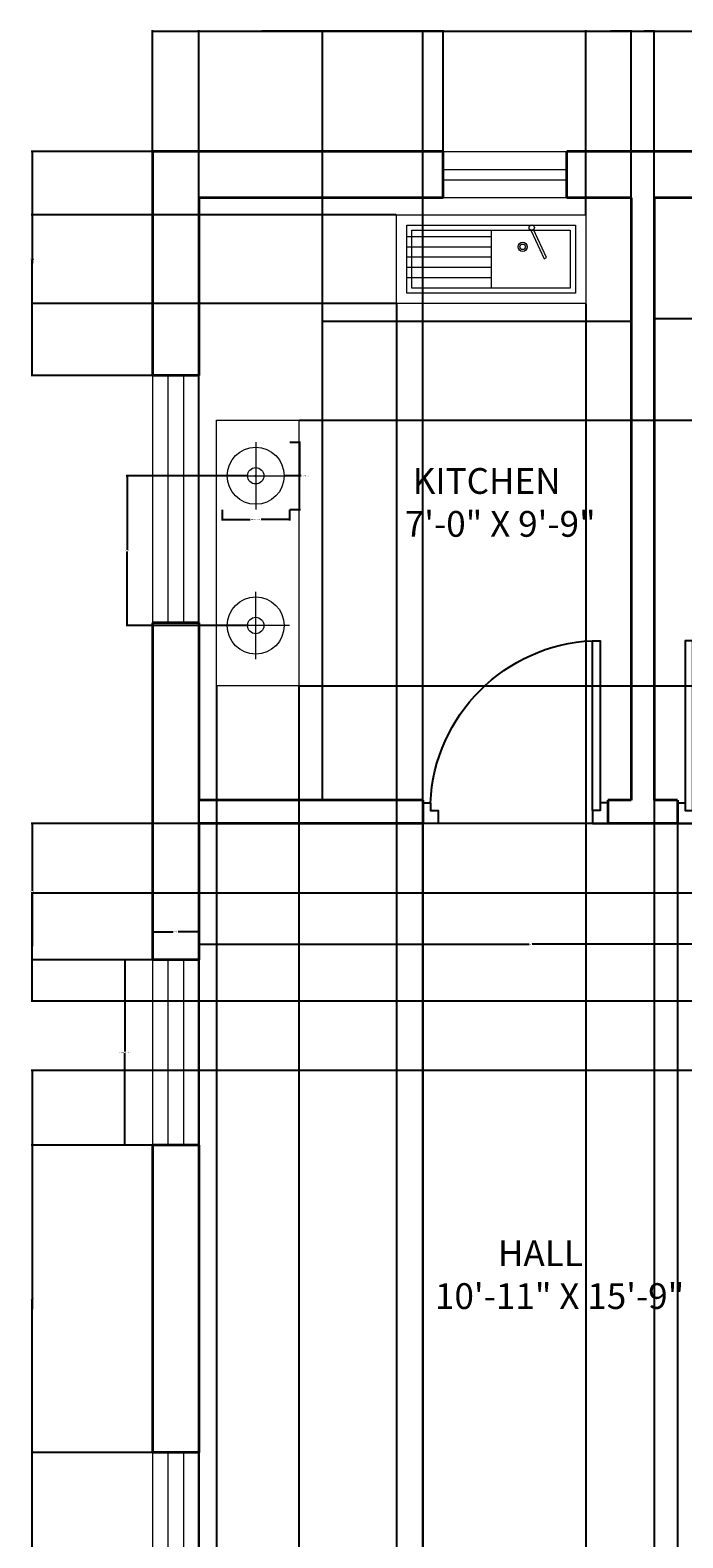
# Model space of a CAD drawing. Units: inches. Extents: x 324 to 662, y 102 to 605.
# Tile 3 of 4: x 324 to 451, y 313 to 605. Entities that reach past the tile are written whole.
import ezdxf

# ---------------------------------------------------------------- set-up
doc = ezdxf.new("R2010")
doc.units = ezdxf.units.IN
for name, color, linetype, lineweight in [('A-ANNO-DIMS', 2, 'Continuous', 18), ('A-AREA-IDEN', 7, 'Continuous', 25), ('A-EQPM', 8, 'Continuous', 18), ('A-FLOR-CASE', 8, 'Continuous', 25), ('A-FLOR-FIXT', 8, 'Continuous', 18), ('door', 82, 'Continuous', 25), ('ventilator', 20, 'Continuous', 18), ('wall', 7, 'Continuous', 35), ('window', 50, 'Continuous', 18)]:
    doc.layers.add(name, color=color, linetype=linetype, lineweight=lineweight)
doc.styles.get("Standard").update_dxf_attribs({"font": 'arial.ttf'})
doc.dimstyles.get("Standard").update_dxf_attribs({"dimtxt": 0.18, "dimasz": 0.18, "dimexe": 0.18, "dimexo": 0.0625, "dimgap": 0.09, "dimtad": 0, "dimtih": 1, "dimtoh": 1, "dimdec": 4, "dimzin": 0, "dimdsep": 46, "dimtxsty": 'Standard', "dimcen": 0.09, "dimadec": 0, "dimazin": 0, "dimtfac": 1, "dimtdec": 4, "dimtofl": 0, "dimtmove": 0, "dimatfit": 3, "dimfxl": 1, "dimtolj": 1, "dimtzin": 0, "dimarcsym": 0})

# ---------------------------------------------------------------- blocks, each defined once
blk = doc.blocks.new('w1')
at = {"layer": 'window'}
for p, q in [((719.66, 290.3), (719.66, 242.3)), ((722.66, 290.3), (722.66, 242.3))]:
    blk.add_line(p, q, dxfattribs=at)
blk.add_lwpolyline([(716.66, 242.3), (725.66, 242.3), (725.66, 290.3), (716.66, 290.3)], close=True, dxfattribs=at)
blk = doc.blocks.new('w2')
at = {"layer": 'window'}
for p, q in [((765.26, 316.2), (765.26, 280.2)), ((768.26, 316.2), (768.26, 280.2))]:
    blk.add_line(p, q, dxfattribs=at)
blk.add_lwpolyline([(762.26, 280.2), (771.26, 280.2), (771.26, 316.2), (762.26, 316.2)], close=True, dxfattribs=at)
blk = doc.blocks.new('d1')
at = {"layer": 'door'}
blk.add_line((825.6, 316.36), (861.6, 316.36), dxfattribs=at)
blk.add_lwpolyline([(827.1, 318.86), (828.6, 318.86), (828.6, 351.86), (827.1, 351.86)], close=True, dxfattribs=at)
for points in [[(828.6, 316.36), (825.6, 316.36), (825.6, 320.36), (827.1, 320.36), (827.1, 318.86), (828.6, 318.86), (828.6, 316.36)], [(858.6, 316.36), (861.6, 316.36), (861.6, 320.36), (860.1, 320.36), (860.1, 318.86), (858.6, 318.86), (858.6, 316.36)]]:
    blk.add_lwpolyline(points, dxfattribs=at)
blk.add_arc((827.1, 318.86), 33.03, 2.6026, 87.3974, dxfattribs=at)
blk = doc.blocks.new('v')
at = {"layer": 'ventilator'}
for p, q in [((1044.91, 377.37), (1044.91, 353.37)), ((1046.91, 377.37), (1046.91, 353.37))]:
    blk.add_line(p, q, dxfattribs=at)
blk.add_lwpolyline([(1041.41, 377.37), (1050.41, 377.37), (1050.41, 353.37), (1041.41, 353.37)], close=True, dxfattribs=at)
blk = doc.blocks.new('COOKTOP-BURNER')
for p, q in [((6.54, 13.08), (6.54, 0)), ((0, 6.54), (13.08, 6.54))]:
    blk.add_line(p, q)
for radius in [5.54, 1.59]:
    blk.add_circle((6.54, 6.54), radius)
blk = doc.blocks.new('*D16')
at = {"layer": 'A-ANNO-DIMS', "color": 0, "lineweight": -2, "transparency": 16777216}
for p, q in [((347.77, 424.9), (342.25, 424.9)), ((342.43, 424.72), (342.43, 407.09)), ((342.43, 389.08), (342.43, 406.72)), ((347.77, 388.9), (342.25, 388.9))]:
    blk.add_line(p, q, dxfattribs=at)
at = {"layer": 'A-ANNO-DIMS', "color": 0, "transparency": 16777216}
for points in [[(342.4, 424.72), (342.46, 424.72), (342.43, 424.9)], [(342.4, 389.08), (342.46, 389.08), (342.43, 388.9)]]:
    blk.add_solid(points, dxfattribs=at)
at = {"layer": 'Defpoints', "color": 0, "transparency": 16777216}
for p in [(342.43, 424.9), (347.83, 424.9), (347.83, 388.9)]:
    blk.add_point(p, dxfattribs=at)
at = {"layer": 'A-ANNO-DIMS', "color": 0, "transparency": 16777216, "insert": (342.43, 406.9), "char_height": 0.18, "attachment_point": 5}
blk.add_mtext('\\A1;WINDOW W2 36 TYP.', dxfattribs=at)
blk = doc.blocks.new('*D17')
at = {"layer": 'A-ANNO-DIMS', "color": 0, "lineweight": -2, "transparency": 16777216}
for p, q in [((347.83, 424.96), (347.83, 430.48)), ((348.01, 430.3), (351.87, 430.3)), ((356.65, 430.3), (352.79, 430.3)), ((356.83, 424.96), (356.83, 430.48))]:
    blk.add_line(p, q, dxfattribs=at)
at = {"layer": 'A-ANNO-DIMS', "color": 0, "transparency": 16777216}
for points in [[(348.01, 430.33), (348.01, 430.27), (347.83, 430.3)], [(356.65, 430.33), (356.65, 430.27), (356.83, 430.3)]]:
    blk.add_solid(points, dxfattribs=at)
at = {"layer": 'Defpoints', "color": 0, "transparency": 16777216}
for p in [(356.83, 430.3), (347.83, 424.9), (356.83, 424.9)]:
    blk.add_point(p, dxfattribs=at)
at = {"layer": 'A-ANNO-DIMS', "color": 0, "transparency": 16777216, "insert": (352.33, 430.3), "char_height": 0.18, "attachment_point": 5}
blk.add_mtext('\\A1;9 TYP.', dxfattribs=at)
blk = doc.blocks.new('*D22')
at = {"layer": 'A-ANNO-DIMS', "color": 0, "lineweight": -2, "transparency": 16777216}
for p, q in [((361.34, 512.29), (361.34, 510.21)), ((361.52, 510.39), (366.79, 510.39)), ((374.24, 510.39), (368.97, 510.39)), ((374.42, 512.29), (374.42, 510.21))]:
    blk.add_line(p, q, dxfattribs=at)
at = {"layer": 'A-ANNO-DIMS', "color": 0, "transparency": 16777216}
for points in [[(361.52, 510.42), (361.52, 510.36), (361.34, 510.39)], [(374.24, 510.42), (374.24, 510.36), (374.42, 510.39)]]:
    blk.add_solid(points, dxfattribs=at)
at = {"layer": 'Defpoints', "color": 0, "transparency": 16777216}
for p in [(361.34, 512.36), (374.42, 512.36), (374.42, 510.39)]:
    blk.add_point(p, dxfattribs=at)
at = {"layer": 'A-ANNO-DIMS', "color": 0, "transparency": 16777216, "insert": (367.88, 510.39), "char_height": 0.18, "attachment_point": 5}
blk.add_mtext('\\A1;BURNER 13 TYP.', dxfattribs=at)
blk = doc.blocks.new('*D23')
at = {"layer": 'A-ANNO-DIMS', "color": 0, "lineweight": -2, "transparency": 16777216}
for p, q in [((374.48, 525.43), (376.56, 525.43)), ((376.38, 525.25), (376.38, 519.08)), ((376.38, 512.54), (376.38, 518.71)), ((374.48, 512.36), (376.56, 512.36))]:
    blk.add_line(p, q, dxfattribs=at)
at = {"layer": 'A-ANNO-DIMS', "color": 0, "transparency": 16777216}
for points in [[(376.35, 525.25), (376.41, 525.25), (376.38, 525.43)], [(376.35, 512.54), (376.41, 512.54), (376.38, 512.36)]]:
    blk.add_solid(points, dxfattribs=at)
at = {"layer": 'Defpoints', "color": 0, "transparency": 16777216}
for p in [(374.42, 525.43), (376.38, 525.43), (374.42, 512.36)]:
    blk.add_point(p, dxfattribs=at)
at = {"layer": 'A-ANNO-DIMS', "color": 0, "transparency": 16777216, "insert": (376.38, 518.9), "char_height": 0.18, "attachment_point": 5}
blk.add_mtext('\\A1;13 TYP.', dxfattribs=at)
blk = doc.blocks.new('*D24')
at = {"layer": 'A-ANNO-DIMS', "color": 0, "lineweight": -2, "transparency": 16777216}
for p, q in [((347.83, 581.92), (347.83, 605.45)), ((348.01, 605.27), (486.04, 605.27)), ((624.65, 605.27), (486.62, 605.27)), ((624.83, 403.42), (624.83, 605.45))]:
    blk.add_line(p, q, dxfattribs=at)
at = {"layer": 'A-ANNO-DIMS', "color": 0, "transparency": 16777216}
for points in [[(348.01, 605.3), (348.01, 605.24), (347.83, 605.27)], [(624.65, 605.3), (624.65, 605.24), (624.83, 605.27)]]:
    blk.add_solid(points, dxfattribs=at)
at = {"layer": 'Defpoints', "color": 0, "transparency": 16777216}
for p in [(624.83, 605.27), (347.83, 581.86), (624.83, 403.36)]:
    blk.add_point(p, dxfattribs=at)
at = {"layer": 'A-ANNO-DIMS', "color": 0, "transparency": 16777216, "insert": (486.33, 605.27), "char_height": 0.18, "attachment_point": 5}
blk.add_mtext('\\A1;277', dxfattribs=at)
blk = doc.blocks.new('*D27')
at = {"layer": 'A-ANNO-DIMS', "color": 0, "lineweight": -2, "transparency": 16777216}
for p, q in [((347.83, 581.92), (347.83, 605.45)), ((348.01, 605.27), (375.68, 605.27)), ((404.14, 605.27), (376.47, 605.27)), ((404.32, 581.92), (404.32, 605.45))]:
    blk.add_line(p, q, dxfattribs=at)
at = {"layer": 'A-ANNO-DIMS', "color": 0, "transparency": 16777216}
for points in [[(348.01, 605.3), (348.01, 605.24), (347.83, 605.27)], [(404.14, 605.3), (404.14, 605.24), (404.32, 605.27)]]:
    blk.add_solid(points, dxfattribs=at)
at = {"layer": 'Defpoints', "color": 0, "transparency": 16777216}
for p in [(404.32, 605.27), (347.83, 581.86), (404.32, 581.86)]:
    blk.add_point(p, dxfattribs=at)
at = {"layer": 'A-ANNO-DIMS', "color": 0, "transparency": 16777216, "insert": (376.07, 605.27), "char_height": 0.18, "attachment_point": 5}
blk.add_mtext('\\A1;56.49', dxfattribs=at)
blk = doc.blocks.new('*D28')
at = {"layer": 'A-ANNO-DIMS', "color": 0, "lineweight": -2, "transparency": 16777216}
for p, q in [((347.77, 581.86), (324.24, 581.86)), ((324.42, 581.68), (324.42, 560.29)), ((324.42, 538.54), (324.42, 559.93)), ((347.77, 538.36), (324.24, 538.36))]:
    blk.add_line(p, q, dxfattribs=at)
at = {"layer": 'A-ANNO-DIMS', "color": 0, "transparency": 16777216}
for points in [[(324.39, 581.68), (324.45, 581.68), (324.42, 581.86)], [(324.39, 538.54), (324.45, 538.54), (324.42, 538.36)]]:
    blk.add_solid(points, dxfattribs=at)
at = {"layer": 'Defpoints', "color": 0, "transparency": 16777216}
for p in [(347.83, 581.86), (324.42, 538.36), (347.83, 538.36)]:
    blk.add_point(p, dxfattribs=at)
at = {"layer": 'A-ANNO-DIMS', "color": 0, "transparency": 16777216, "insert": (324.42, 560.11), "char_height": 0.18, "attachment_point": 5}
blk.add_mtext('\\A1;43.5', dxfattribs=at)
blk = doc.blocks.new('*D29')
at = {"layer": 'A-ANNO-DIMS', "color": 0, "lineweight": -2, "transparency": 16777216}
for p, q in [((356.77, 451.36), (324.24, 451.36)), ((324.42, 451.18), (324.42, 438.31)), ((324.42, 425.08), (324.42, 437.95)), ((356.77, 424.9), (324.24, 424.9))]:
    blk.add_line(p, q, dxfattribs=at)
at = {"layer": 'A-ANNO-DIMS', "color": 0, "transparency": 16777216}
for points in [[(324.39, 451.18), (324.45, 451.18), (324.42, 451.36)], [(324.39, 425.08), (324.45, 425.08), (324.42, 424.9)]]:
    blk.add_solid(points, dxfattribs=at)
at = {"layer": 'Defpoints', "color": 0, "transparency": 16777216}
for p in [(356.83, 451.36), (324.42, 424.9), (356.83, 424.9)]:
    blk.add_point(p, dxfattribs=at)
at = {"layer": 'A-ANNO-DIMS', "color": 0, "transparency": 16777216, "insert": (324.42, 438.13), "char_height": 0.18, "attachment_point": 5}
blk.add_mtext('\\A1;26.46', dxfattribs=at)
blk = doc.blocks.new('*D30')
at = {"layer": 'A-ANNO-DIMS', "color": 0, "lineweight": -2, "transparency": 16777216}
for p, q in [((347.77, 388.9), (324.24, 388.9)), ((324.42, 388.72), (324.42, 359.24)), ((324.42, 329.39), (324.42, 358.88)), ((347.77, 329.21), (324.24, 329.21))]:
    blk.add_line(p, q, dxfattribs=at)
at = {"layer": 'A-ANNO-DIMS', "color": 0, "transparency": 16777216}
for points in [[(324.39, 388.72), (324.45, 388.72), (324.42, 388.9)], [(324.39, 329.39), (324.45, 329.39), (324.42, 329.21)]]:
    blk.add_solid(points, dxfattribs=at)
at = {"layer": 'Defpoints', "color": 0, "transparency": 16777216}
for p in [(347.83, 388.9), (324.42, 329.21), (347.83, 329.21)]:
    blk.add_point(p, dxfattribs=at)
at = {"layer": 'A-ANNO-DIMS', "color": 0, "transparency": 16777216, "insert": (324.42, 359.06), "char_height": 0.18, "attachment_point": 5}
blk.add_mtext('\\A1;59.69', dxfattribs=at)
blk = doc.blocks.new('*D34')
at = {"layer": 'A-ANNO-DIMS', "color": 0, "lineweight": -2, "transparency": 16777216}
for p, q in [((490.27, 403.36), (324.24, 403.36)), ((324.42, 403.18), (324.42, 357.04)), ((324.42, 310.54), (324.42, 356.68)), ((490.27, 310.36), (324.24, 310.36))]:
    blk.add_line(p, q, dxfattribs=at)
at = {"layer": 'A-ANNO-DIMS', "color": 0, "transparency": 16777216}
for points in [[(324.39, 403.18), (324.45, 403.18), (324.42, 403.36)], [(324.39, 310.54), (324.45, 310.54), (324.42, 310.36)]]:
    blk.add_solid(points, dxfattribs=at)
at = {"layer": 'Defpoints', "color": 0, "transparency": 16777216}
for p in [(490.33, 403.36), (324.42, 310.36), (490.33, 310.36)]:
    blk.add_point(p, dxfattribs=at)
at = {"layer": 'A-ANNO-DIMS', "color": 0, "transparency": 16777216, "insert": (324.42, 356.86), "char_height": 0.18, "attachment_point": 5}
blk.add_mtext('\\A1;93', dxfattribs=at)
blk = doc.blocks.new('*D39')
at = {"layer": 'A-ANNO-DIMS', "color": 0, "lineweight": -2, "transparency": 16777216}
for p, q in [((356.83, 166.92), (356.83, 605.45)), ((357.01, 605.27), (378.25, 605.27)), ((400.15, 605.27), (378.91, 605.27)), ((400.33, 166.92), (400.33, 605.45))]:
    blk.add_line(p, q, dxfattribs=at)
at = {"layer": 'A-ANNO-DIMS', "color": 0, "transparency": 16777216}
for points in [[(357.01, 605.3), (357.01, 605.24), (356.83, 605.27)], [(400.15, 605.3), (400.15, 605.24), (400.33, 605.27)]]:
    blk.add_solid(points, dxfattribs=at)
at = {"layer": 'Defpoints', "color": 0, "transparency": 16777216}
for p in [(400.33, 605.27), (356.83, 166.86), (400.33, 166.86)]:
    blk.add_point(p, dxfattribs=at)
at = {"layer": 'A-ANNO-DIMS', "color": 0, "transparency": 16777216, "insert": (378.58, 605.27), "char_height": 0.18, "attachment_point": 5}
blk.add_mtext('\\A1;43.5', dxfattribs=at)
blk = doc.blocks.new('*D42')
at = {"layer": 'A-ANNO-DIMS', "color": 0, "lineweight": -2, "transparency": 16777216}
for p, q in [((440.83, 572.92), (440.83, 605.45)), ((441.01, 605.27), (442.82, 605.27)), ((445.15, 605.27), (443.34, 605.27)), ((445.33, 572.92), (445.33, 605.45))]:
    blk.add_line(p, q, dxfattribs=at)
at = {"layer": 'A-ANNO-DIMS', "color": 0, "transparency": 16777216}
for points in [[(441.01, 605.3), (441.01, 605.24), (440.83, 605.27)], [(445.15, 605.3), (445.15, 605.24), (445.33, 605.27)]]:
    blk.add_solid(points, dxfattribs=at)
at = {"layer": 'Defpoints', "color": 0, "transparency": 16777216}
for p in [(445.33, 605.27), (440.83, 572.86), (445.33, 572.86)]:
    blk.add_point(p, dxfattribs=at)
at = {"layer": 'A-ANNO-DIMS', "color": 0, "transparency": 16777216, "insert": (443.08, 605.27), "char_height": 0.18, "attachment_point": 5}
blk.add_mtext('\\A1;4.5', dxfattribs=at)
blk = doc.blocks.new('*D43')
at = {"layer": 'A-ANNO-DIMS', "color": 0, "lineweight": -2, "transparency": 16777216}
for p, q in [((356.83, 455.92), (356.83, 605.45)), ((357.01, 605.27), (368.61, 605.27)), ((380.65, 605.27), (369.05, 605.27)), ((380.83, 455.92), (380.83, 605.45))]:
    blk.add_line(p, q, dxfattribs=at)
at = {"layer": 'A-ANNO-DIMS', "color": 0, "transparency": 16777216}
for points in [[(357.01, 605.3), (357.01, 605.24), (356.83, 605.27)], [(380.65, 605.3), (380.65, 605.24), (380.83, 605.27)]]:
    blk.add_solid(points, dxfattribs=at)
at = {"layer": 'Defpoints', "color": 0, "transparency": 16777216}
for p in [(380.83, 605.27), (356.83, 455.86), (380.83, 455.86)]:
    blk.add_point(p, dxfattribs=at)
at = {"layer": 'A-ANNO-DIMS', "color": 0, "transparency": 16777216, "insert": (368.83, 605.27), "char_height": 0.18, "attachment_point": 5}
blk.add_mtext('\\A1;24', dxfattribs=at)
blk = doc.blocks.new('*D48')
at = {"layer": 'A-ANNO-DIMS', "color": 0, "lineweight": -2, "transparency": 16777216}
for p, q in [((395.24, 552.3), (395.24, 102.17)), ((432.02, 552.3), (432.02, 102.17)), ((395.42, 102.35), (413.24, 102.35)), ((431.84, 102.35), (414.02, 102.35))]:
    blk.add_line(p, q, dxfattribs=at)
at = {"layer": 'A-ANNO-DIMS', "color": 0, "transparency": 16777216}
for points in [[(395.42, 102.38), (395.42, 102.32), (395.24, 102.35)], [(431.84, 102.38), (431.84, 102.32), (432.02, 102.35)]]:
    blk.add_solid(points, dxfattribs=at)
at = {"layer": 'Defpoints', "color": 0, "transparency": 16777216}
for p in [(395.24, 552.36), (432.02, 552.36), (432.02, 102.35)]:
    blk.add_point(p, dxfattribs=at)
at = {"layer": 'A-ANNO-DIMS', "color": 0, "transparency": 16777216, "insert": (413.63, 102.35), "char_height": 0.18, "attachment_point": 5}
blk.add_mtext('\\A1;36.79', dxfattribs=at)
blk = doc.blocks.new('*D49')
at = {"layer": 'A-ANNO-DIMS', "color": 0, "lineweight": -2, "transparency": 16777216}
for p, q in [((395.17, 569.61), (324.24, 569.61)), ((324.42, 569.43), (324.42, 561.16)), ((324.42, 552.54), (324.42, 560.8)), ((395.17, 552.36), (324.24, 552.36))]:
    blk.add_line(p, q, dxfattribs=at)
at = {"layer": 'A-ANNO-DIMS', "color": 0, "transparency": 16777216}
for points in [[(324.39, 569.43), (324.45, 569.43), (324.42, 569.61)], [(324.39, 552.54), (324.45, 552.54), (324.42, 552.36)]]:
    blk.add_solid(points, dxfattribs=at)
at = {"layer": 'Defpoints', "color": 0, "transparency": 16777216}
for p in [(324.42, 569.61), (395.24, 569.61), (395.24, 552.36)]:
    blk.add_point(p, dxfattribs=at)
at = {"layer": 'A-ANNO-DIMS', "color": 0, "transparency": 16777216, "insert": (324.42, 560.98), "char_height": 0.18, "attachment_point": 5}
blk.add_mtext('\\A1;17.246', dxfattribs=at)
blk = doc.blocks.new('*D50')
at = {"layer": 'A-ANNO-DIMS', "color": 0, "lineweight": -2, "transparency": 16777216}
for p, q in [((445.33, 572.8), (445.33, 549.26)), ((483.08, 572.8), (483.08, 549.26)), ((445.51, 549.44), (463.74, 549.44)), ((482.9, 549.44), (464.67, 549.44))]:
    blk.add_line(p, q, dxfattribs=at)
at = {"layer": 'A-ANNO-DIMS', "color": 0, "transparency": 16777216}
for points in [[(445.51, 549.47), (445.51, 549.41), (445.33, 549.44)], [(482.9, 549.47), (482.9, 549.41), (483.08, 549.44)]]:
    blk.add_solid(points, dxfattribs=at)
at = {"layer": 'Defpoints', "color": 0, "transparency": 16777216}
for p in [(445.33, 572.86), (483.08, 572.86), (445.33, 549.44)]:
    blk.add_point(p, dxfattribs=at)
at = {"layer": 'A-ANNO-DIMS', "color": 0, "transparency": 16777216, "insert": (464.21, 549.44), "char_height": 0.18, "attachment_point": 5}
blk.add_mtext('\\A1;37.754', dxfattribs=at)
blk = doc.blocks.new('*D51')
at = {"layer": 'A-ANNO-DIMS', "color": 0, "lineweight": -2, "transparency": 16777216}
for p, q in [((356.83, 455.8), (356.83, 102.17)), ((400.33, 455.8), (400.33, 102.17)), ((357.01, 102.35), (378.25, 102.35)), ((400.15, 102.35), (378.91, 102.35))]:
    blk.add_line(p, q, dxfattribs=at)
at = {"layer": 'A-ANNO-DIMS', "color": 0, "transparency": 16777216}
for points in [[(357.01, 102.38), (357.01, 102.32), (356.83, 102.35)], [(400.15, 102.38), (400.15, 102.32), (400.33, 102.35)]]:
    blk.add_solid(points, dxfattribs=at)
at = {"layer": 'Defpoints', "color": 0, "transparency": 16777216}
for p in [(356.83, 455.86), (400.33, 455.86), (400.33, 102.35)]:
    blk.add_point(p, dxfattribs=at)
at = {"layer": 'A-ANNO-DIMS', "color": 0, "transparency": 16777216, "insert": (378.58, 102.35), "char_height": 0.18, "attachment_point": 5}
blk.add_mtext('\\A1;43.5', dxfattribs=at)
blk = doc.blocks.new('*D52')
at = {"layer": 'A-ANNO-DIMS', "color": 0, "lineweight": -2, "transparency": 16777216}
for p, q in [((445.33, 455.8), (445.33, 102.17)), ((449.83, 451.3), (449.83, 102.17)), ((445.51, 102.35), (447.32, 102.35)), ((449.65, 102.35), (447.84, 102.35))]:
    blk.add_line(p, q, dxfattribs=at)
at = {"layer": 'A-ANNO-DIMS', "color": 0, "transparency": 16777216}
for points in [[(445.51, 102.38), (445.51, 102.32), (445.33, 102.35)], [(449.65, 102.38), (449.65, 102.32), (449.83, 102.35)]]:
    blk.add_solid(points, dxfattribs=at)
at = {"layer": 'Defpoints', "color": 0, "transparency": 16777216}
for p in [(445.33, 455.86), (449.83, 451.36), (449.83, 102.35)]:
    blk.add_point(p, dxfattribs=at)
at = {"layer": 'A-ANNO-DIMS', "color": 0, "transparency": 16777216, "insert": (447.58, 102.35), "char_height": 0.18, "attachment_point": 5}
blk.add_mtext('\\A1;4.5', dxfattribs=at)
blk = doc.blocks.new('*D57')
at = {"layer": 'A-ANNO-DIMS', "color": 0, "lineweight": -2, "transparency": 16777216}
for p, q in [((570.77, 437.86), (324.24, 437.86)), ((324.42, 437.68), (324.42, 427.54)), ((324.42, 417.04), (324.42, 427.18)), ((570.77, 416.86), (324.24, 416.86))]:
    blk.add_line(p, q, dxfattribs=at)
at = {"layer": 'A-ANNO-DIMS', "color": 0, "transparency": 16777216}
for points in [[(324.39, 437.68), (324.45, 437.68), (324.42, 437.86)], [(324.39, 417.04), (324.45, 417.04), (324.42, 416.86)]]:
    blk.add_solid(points, dxfattribs=at)
at = {"layer": 'Defpoints', "color": 0, "transparency": 16777216}
for p in [(324.42, 437.86), (570.83, 437.86), (570.83, 416.86)]:
    blk.add_point(p, dxfattribs=at)
at = {"layer": 'A-ANNO-DIMS', "color": 0, "transparency": 16777216, "insert": (324.42, 427.36), "char_height": 0.18, "attachment_point": 5}
blk.add_mtext('\\A1;21', dxfattribs=at)
blk = doc.blocks.new('*D59')
at = {"layer": 'A-ANNO-DIMS', "color": 0, "lineweight": -2, "transparency": 16777216}
for p, q in [((360.27, 478.01), (360.27, 102.17)), ((376.24, 478.01), (376.24, 102.17)), ((360.45, 102.35), (367.87, 102.35)), ((376.06, 102.35), (368.64, 102.35))]:
    blk.add_line(p, q, dxfattribs=at)
at = {"layer": 'A-ANNO-DIMS', "color": 0, "transparency": 16777216}
for points in [[(360.45, 102.38), (360.45, 102.32), (360.27, 102.35)], [(376.06, 102.38), (376.06, 102.32), (376.24, 102.35)]]:
    blk.add_solid(points, dxfattribs=at)
at = {"layer": 'Defpoints', "color": 0, "transparency": 16777216}
for p in [(360.27, 478.07), (376.24, 478.07), (376.24, 102.35)]:
    blk.add_point(p, dxfattribs=at)
at = {"layer": 'A-ANNO-DIMS', "color": 0, "transparency": 16777216, "insert": (368.25, 102.35), "char_height": 0.18, "attachment_point": 5}
blk.add_mtext('\\A1;15.97', dxfattribs=at)
blk = doc.blocks.new('*D60')
at = {"layer": 'A-ANNO-DIMS', "color": 0, "lineweight": -2, "transparency": 16777216}
for p, q in [((376.3, 529.67), (662.43, 529.67)), ((662.25, 529.49), (662.25, 504.05)), ((662.25, 478.25), (662.25, 503.69)), ((376.3, 478.07), (662.43, 478.07))]:
    blk.add_line(p, q, dxfattribs=at)
at = {"layer": 'A-ANNO-DIMS', "color": 0, "transparency": 16777216}
for points in [[(662.22, 529.49), (662.28, 529.49), (662.25, 529.67)], [(662.22, 478.25), (662.28, 478.25), (662.25, 478.07)]]:
    blk.add_solid(points, dxfattribs=at)
at = {"layer": 'Defpoints', "color": 0, "transparency": 16777216}
for p in [(376.24, 529.67), (662.25, 529.67), (376.24, 478.07)]:
    blk.add_point(p, dxfattribs=at)
at = {"layer": 'A-ANNO-DIMS', "color": 0, "transparency": 16777216, "insert": (662.25, 503.87), "char_height": 0.18, "attachment_point": 5}
blk.add_mtext('\\A1;51.6', dxfattribs=at)
blk = doc.blocks.new('*D62')
at = {"layer": 'A-ANNO-DIMS', "color": 0, "lineweight": -2, "transparency": 16777216}
for p, q in [((356.83, 451.3), (356.83, 427.76)), ((485.83, 451.3), (485.83, 427.76)), ((357.01, 427.94), (421.05, 427.94)), ((485.65, 427.94), (421.61, 427.94))]:
    blk.add_line(p, q, dxfattribs=at)
at = {"layer": 'A-ANNO-DIMS', "color": 0, "transparency": 16777216}
for points in [[(357.01, 427.97), (357.01, 427.91), (356.83, 427.94)], [(485.65, 427.97), (485.65, 427.91), (485.83, 427.94)]]:
    blk.add_solid(points, dxfattribs=at)
at = {"layer": 'Defpoints', "color": 0, "transparency": 16777216}
for p in [(356.83, 451.36), (485.83, 451.36), (356.83, 427.94)]:
    blk.add_point(p, dxfattribs=at)
at = {"layer": 'A-ANNO-DIMS', "color": 0, "transparency": 16777216, "insert": (421.33, 427.94), "char_height": 0.18, "attachment_point": 5}
blk.add_mtext('\\A1;129', dxfattribs=at)
blk = doc.blocks.new('*D66')
at = {"layer": 'A-ANNO-DIMS', "color": 0, "lineweight": -2, "transparency": 16777216}
for p, q in [((432.02, 569.67), (432.02, 605.45)), ((432.2, 605.27), (436.03, 605.27)), ((440.65, 605.27), (436.82, 605.27)), ((440.83, 572.92), (440.83, 605.45))]:
    blk.add_line(p, q, dxfattribs=at)
at = {"layer": 'A-ANNO-DIMS', "color": 0, "transparency": 16777216}
for points in [[(432.2, 605.3), (432.2, 605.24), (432.02, 605.27)], [(440.65, 605.3), (440.65, 605.24), (440.83, 605.27)]]:
    blk.add_solid(points, dxfattribs=at)
at = {"layer": 'Defpoints', "color": 0, "transparency": 16777216}
for p in [(440.83, 605.27), (440.83, 572.86), (432.02, 569.61)]:
    blk.add_point(p, dxfattribs=at)
at = {"layer": 'A-ANNO-DIMS', "color": 0, "transparency": 16777216, "insert": (436.43, 605.27), "char_height": 0.18, "attachment_point": 5}
blk.add_mtext('\\A1;8.807', dxfattribs=at)
blk = doc.blocks.new('*D67')
at = {"layer": 'A-ANNO-DIMS', "color": 0, "lineweight": -2, "transparency": 16777216}
for p, q in [((366.23, 518.9), (342.7, 518.9)), ((342.88, 518.72), (342.88, 504.54)), ((342.88, 490), (342.88, 504.17)), ((366.23, 489.82), (342.7, 489.82))]:
    blk.add_line(p, q, dxfattribs=at)
at = {"layer": 'A-ANNO-DIMS', "color": 0, "transparency": 16777216}
for points in [[(342.85, 518.72), (342.91, 518.72), (342.88, 518.9)], [(342.85, 490), (342.91, 490), (342.88, 489.82)]]:
    blk.add_solid(points, dxfattribs=at)
at = {"layer": 'Defpoints', "color": 0, "transparency": 16777216}
for p in [(342.88, 518.9), (366.29, 518.9), (366.29, 489.82)]:
    blk.add_point(p, dxfattribs=at)
at = {"layer": 'A-ANNO-DIMS', "color": 0, "transparency": 16777216, "insert": (342.88, 504.36), "char_height": 0.18, "attachment_point": 5}
blk.add_mtext('\\A1;29.08', dxfattribs=at)
blk = doc.blocks.new('*D70')
at = {"layer": 'A-ANNO-DIMS', "color": 0, "lineweight": -2, "transparency": 16777216}
for p, q in [((367.79, 518.9), (367.97, 518.9)), ((367.88, 518.81), (367.88, 518.99)), ((376.74, 518.89), (373.6, 518.89))]:
    blk.add_line(p, q, dxfattribs=at)
at = {"layer": 'A-ANNO-DIMS', "color": 0, "transparency": 16777216}
blk.add_solid([(373.6, 518.92), (373.6, 518.86), (373.42, 518.89)], dxfattribs=at)
at = {"layer": 'Defpoints', "color": 0, "transparency": 16777216}
for p in [(362.34, 518.9), (373.42, 518.89)]:
    blk.add_point(p, dxfattribs=at)
at = {"layer": 'A-ANNO-DIMS', "color": 0, "transparency": 16777216, "insert": (377.5, 518.89), "char_height": 0.18, "attachment_point": 5}
blk.add_mtext('\\A1;2X ∅11.078', dxfattribs=at)

msp = doc.modelspace()

# ---------------------------------------------------------------- linework, layer by layer
at = {"layer": 'A-EQPM'}
msp.add_lwpolyline([(360.2695, 529.67), (376.2379, 529.67), (376.2379, 478.07), (360.2695, 478.07)], close=True, dxfattribs=at)
at = {"layer": 'A-FLOR-CASE'}
for p in [(380.8304, 455.8598), (440.8304, 548.8598)]:
    msp.add_line(p, (380.8304, 548.8598), dxfattribs=at)
at = {"layer": 'A-FLOR-FIXT'}
for p, q in [((413.6295, 565.3343), (397.2356, 565.3343)), ((413.6295, 566.6051), (413.6295, 555.3588)), ((413.6295, 563.3343), (397.2356, 563.3343)), ((413.6295, 561.3343), (397.2356, 561.3343)), ((413.6295, 559.3343), (397.2356, 559.3343)), ((413.6295, 557.3343), (397.2356, 557.3343))]:
    msp.add_line(p, q, dxfattribs=at)
for points in [[(395.2356, 569.6051), (432.0233, 569.6051), (432.0233, 552.3588), (395.2356, 552.3588)], [(397.2356, 567.6051), (430.0233, 567.6051), (430.0233, 554.3588), (397.2356, 554.3588)], [(398.2356, 566.6051), (429.0233, 566.6051), (429.0233, 555.3588), (398.2356, 555.3588)], [(423.9153, 561.0546), (424.3691, 561.2645), (421.8502, 566.7101), (421.3964, 566.5002)]]:
    msp.add_lwpolyline(points, close=True, dxfattribs=at)
for centre, radius in [((421.5272, 567.1101), 0.5141), ((419.764, 563.3614), 0.8926), ((419.764, 563.3614), 0.541)]:
    msp.add_circle(centre, radius, dxfattribs=at)
at = {"layer": 'wall'}
for p, q in [((347.8304, 581.8598), (347.8304, 538.3598)), ((404.3193, 581.8598), (347.8304, 581.8598)), ((404.3193, 572.8598), (404.3193, 581.8598)), ((587.8304, 581.8598), (428.3193, 581.8598)), ((428.3193, 572.8598), (428.3193, 581.8598)), ((356.8304, 572.8598), (356.8304, 538.3598)), ((404.3193, 572.8598), (356.8304, 572.8598)), ((440.8304, 572.8598), (428.3193, 572.8598)), ((440.8304, 572.8598), (440.8304, 455.8598)), ((578.8304, 572.8598), (445.3304, 572.8598)), ((445.3304, 572.8598), (445.3304, 455.8598)), ((356.8304, 538.3598), (347.8304, 538.3598)), ((356.8304, 490.3598), (347.8304, 490.3598)), ((347.8304, 490.3598), (347.8304, 424.9021)), ((356.8304, 490.3598), (356.8304, 455.8598)), ((400.3304, 455.8598), (356.8304, 455.8598)), ((400.3304, 455.8598), (400.3304, 451.3598)), ((440.8304, 455.8598), (436.3304, 455.8598)), ((436.3304, 455.8598), (436.3304, 451.3598)), ((449.8304, 455.8598), (445.3304, 455.8598)), ((449.8304, 455.8598), (449.8304, 451.3598)), ((356.8304, 451.3598), (356.8304, 424.9021)), ((400.3304, 451.3598), (356.8304, 451.3598)), ((449.8304, 451.3598), (436.3304, 451.3598)), ((356.8304, 424.9021), (347.8304, 424.9021)), ((356.8304, 388.9021), (347.8304, 388.9021)), ((347.8304, 388.9021), (347.8304, 329.2144)), ((356.8304, 388.9021), (356.8304, 329.2144)), ((356.8304, 329.2144), (347.8304, 329.2144))]:
    msp.add_line(p, q, dxfattribs=at)

# ---------------------------------------------------------------- block references
at = {"layer": 'A-EQPM'}
msp.add_blockref('COOKTOP-BURNER', (361.343, 512.356), dxfattribs=at)
at = {"layer": 'A-EQPM', "rotation": 180}
msp.add_blockref('COOKTOP-BURNER', (374.4205, 496.3559), dxfattribs=at)
at = {"layer": 'door', "xscale": -1}
msp.add_blockref('d1', (1261.935, 135.0041), dxfattribs=at)
at = {"layer": 'door'}
msp.add_blockref('d1', (-375.7743, 135.0041), dxfattribs=at)
at = {"layer": 'ventilator', "rotation": 90}
msp.add_blockref('v', (781.6926, -468.5481), dxfattribs=at)
at = {"layer": 'window'}
for name, p in [('w1', (-368.8269, 248.0552)), ('w2', (-414.4328, 108.7023)), ('w2', (-414.4328, 13.0146))]:
    msp.add_blockref(name, p, dxfattribs=at)

# ---------------------------------------------------------------- texts
at = {"layer": 'A-AREA-IDEN', "char_height": 5, "attachment_point": 1}
for s, insert in [(' KITCHEN\\P7\'-0" X 9\'-9"', (396.8525, 520.389)), ('        HALL\\P10\'-11" X 15\'-9"', (402.7164, 370.4))]:
    msp.add_mtext_dynamic_manual_height_columns(s, width=50.156641, gutter_width=12.5, heights=[0], dxfattribs=dict(at, insert=insert))

# ---------------------------------------------------------------- dimensions: what is measured, and where the dimension line sits
at = {"layer": 'A-ANNO-DIMS'}
for base, p1, p2, override, picture, middle in [((624.8304, 605.2748), (347.8304, 581.8598), (624.8304, 403.3598), {"dimdec": 0, "dimlfac": 1, "dimrnd": 0, "dimzin": 0, "dimdsep": 46, "dimlunit": 2}, '*D24', (486.3304, 605.2748)), ((404.3193, 605.2748), (347.8304, 581.8598), (404.3193, 581.8598), {"dimdec": 2, "dimlfac": 1, "dimrnd": 0, "dimzin": 0, "dimdsep": 46, "dimlunit": 2}, '*D27', (376.0749, 605.2748)), ((400.3304, 605.2748), (356.8304, 166.8598), (400.3304, 166.8598), {"dimdec": 1, "dimlfac": 1, "dimrnd": 0, "dimzin": 0, "dimdsep": 46, "dimlunit": 2}, '*D39', (378.5804, 605.2748)), ((380.8304, 605.2748), (356.8304, 455.8598), (380.8304, 455.8598), {"dimdec": 0, "dimlfac": 1, "dimrnd": 0, "dimzin": 0, "dimdsep": 46, "dimlunit": 2}, '*D43', (368.8304, 605.2748)), ((440.8304, 605.2748), (432.0233, 569.6051), (440.8304, 572.8598), {"dimdec": 3, "dimlfac": 1, "dimrnd": 0, "dimzin": 0, "dimdsep": 46, "dimlunit": 2}, '*D66', (436.4268, 605.2748)), ((445.3304, 605.2748), (440.8304, 572.8598), (445.3304, 572.8598), {"dimdec": 1, "dimlfac": 1, "dimrnd": 0, "dimzin": 0, "dimdsep": 46, "dimlunit": 2}, '*D42', (443.0804, 605.2748)), ((432.0233, 102.3527), (395.2356, 552.3588), (432.0233, 552.3588), {"dimdec": 2, "dimlfac": 1, "dimrnd": 0, "dimzin": 0, "dimdsep": 46, "dimlunit": 2}, '*D48', (413.6295, 102.3527)), ((376.2379, 102.3527), (360.2695, 478.07), (376.2379, 478.07), {"dimdec": 2, "dimlfac": 1, "dimrnd": 0, "dimzin": 0, "dimdsep": 46, "dimlunit": 2}, '*D59', (368.2537, 102.3527)), ((400.3304, 102.3527), (356.8304, 455.8598), (400.3304, 455.8598), {"dimdec": 1, "dimlfac": 1, "dimrnd": 0, "dimzin": 0, "dimdsep": 46, "dimlunit": 2}, '*D51', (378.5804, 102.3527)), ((449.8304, 102.3527), (445.3304, 455.8598), (449.8304, 451.3598), {"dimdec": 1, "dimlfac": 1, "dimrnd": 0, "dimzin": 0, "dimdsep": 46, "dimlunit": 2}, '*D52', (447.5804, 102.3527))]:
    dim = msp.add_linear_dim(base=base, p1=p1, p2=p2, dimstyle='Standard', override=override, dxfattribs=at)
    dim.commit()
    dim.dimension.update_dxf_attribs({"geometry": picture, "text_midpoint": middle})
for base, p1, p2, angle, override, picture, middle in [((324.4154, 538.3598), (347.8304, 581.8598), (347.8304, 538.3598), 90, {"dimdec": 1, "dimlfac": 1, "dimrnd": 0, "dimzin": 0, "dimdsep": 46, "dimlunit": 2}, '*D28', (324.4154, 560.1098)), ((445.3304, 549.4448), (483.0848, 572.8598), (445.3304, 572.8598), 180, {"dimdec": 3, "dimlfac": 1, "dimrnd": 0, "dimzin": 0, "dimdsep": 46, "dimlunit": 2}, '*D50', (464.2076, 549.4448)), ((324.4154, 569.6051), (395.2356, 552.3588), (395.2356, 569.6051), 90, {"dimdec": 3, "dimlfac": 1, "dimrnd": 0, "dimzin": 0, "dimdsep": 46, "dimlunit": 2}, '*D49', (324.4154, 560.982)), ((662.2454, 529.67), (376.2379, 478.07), (376.2379, 529.67), 90, {"dimdec": 1, "dimlfac": 1, "dimrnd": 0, "dimzin": 0, "dimdsep": 46, "dimlunit": 2}, '*D60', (662.2454, 503.87)), ((342.8776, 518.8953), (366.2926, 489.8167), (366.2926, 518.8953), 90, {"dimdec": 2, "dimlfac": 1, "dimrnd": 0, "dimzin": 0, "dimdsep": 46, "dimlunit": 2}, '*D67', (342.8776, 504.356)), ((324.4154, 424.9021), (356.8304, 451.3598), (356.8304, 424.9021), 90, {"dimdec": 2, "dimlfac": 1, "dimrnd": 0, "dimzin": 0, "dimdsep": 46, "dimlunit": 2}, '*D29', (324.4154, 438.1309)), ((356.8304, 427.9448), (485.8304, 451.3598), (356.8304, 451.3598), 180, {"dimdec": 0, "dimlfac": 1, "dimrnd": 0, "dimzin": 0, "dimdsep": 46, "dimlunit": 2}, '*D62', (421.3304, 427.9448)), ((324.4154, 437.8598), (570.8304, 416.8598), (570.8304, 437.8598), 90, {"dimdec": 0, "dimlfac": 1, "dimrnd": 0, "dimzin": 0, "dimdsep": 46, "dimlunit": 2}, '*D57', (324.4154, 427.3598)), ((324.4154, 310.3598), (490.3304, 403.3598), (490.3304, 310.3598), 90, {"dimdec": 0, "dimlfac": 1, "dimrnd": 0, "dimzin": 0, "dimdsep": 46, "dimlunit": 2}, '*D34', (324.4154, 356.8598)), ((324.4154, 329.2144), (347.8304, 388.9021), (347.8304, 329.2144), 90, {"dimdec": 2, "dimlfac": 1, "dimrnd": 0, "dimzin": 0, "dimdsep": 46, "dimlunit": 2}, '*D30', (324.4154, 359.0582))]:
    dim = msp.add_linear_dim(base=base, p1=p1, p2=p2, angle=angle, dimstyle='Standard', override=override, dxfattribs=at)
    dim.commit()
    dim.dimension.update_dxf_attribs({"geometry": picture, "text_midpoint": middle})
for base, p1, p2, text, picture, middle in [((376.3821, 525.434), (374.4205, 512.3565), (374.4205, 525.434), '<> TYP.', '*D23', (376.3821, 518.8953)), ((342.4304, 424.9021), (347.8304, 388.9021), (347.8304, 424.9021), 'WINDOW W2 <> TYP.', '*D16', (342.4304, 406.9021))]:
    dim = msp.add_linear_dim(base=base, p1=p1, p2=p2, angle=90, text=text, dimstyle='Standard', override={"dimdec": 0, "dimlfac": 1, "dimrnd": 0, "dimzin": 0, "dimdsep": 46, "dimlunit": 2}, dxfattribs=at)
    dim.commit()
    dim.dimension.update_dxf_attribs({"geometry": picture, "text_midpoint": middle})
dim = msp.add_diameter_dim_2p(p1=(362.3429, 518.8955), p2=(373.4205, 518.895), text='2X <>', dimstyle='Standard', override={"dimdec": 3, "dimlfac": 1, "dimrnd": 0, "dimzin": 0, "dimdsep": 46, "dimlunit": 2}, dxfattribs=at)
dim.commit()
dim.dimension.update_dxf_attribs({"geometry": '*D70', "text_midpoint": (376.7438, 518.8948), "dimtype": 163})
for base, p1, p2, text, picture, middle in [((374.4205, 510.3948), (361.3429, 512.3565), (374.4205, 512.3565), 'BURNER <> TYP.', '*D22', (367.8817, 510.3948)), ((356.8304, 430.3021), (347.8304, 424.9021), (356.8304, 424.9021), '<> TYP.', '*D17', (352.3304, 430.3021))]:
    dim = msp.add_linear_dim(base=base, p1=p1, p2=p2, text=text, dimstyle='Standard', override={"dimdec": 0, "dimlfac": 1, "dimrnd": 0, "dimzin": 0, "dimdsep": 46, "dimlunit": 2}, dxfattribs=at)
    dim.commit()
    dim.dimension.update_dxf_attribs({"geometry": picture, "text_midpoint": middle})

doc.saveas('drawing.dxf')
